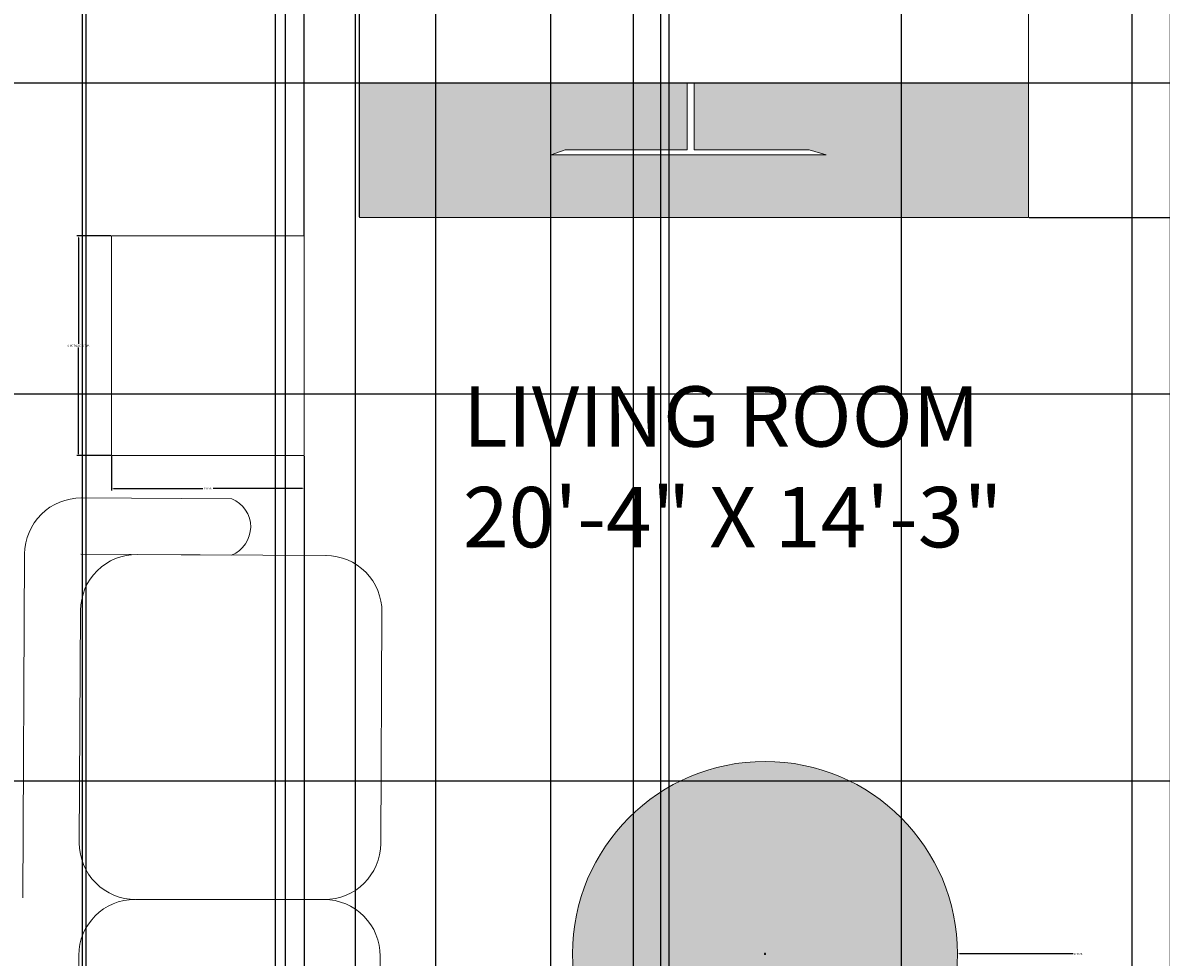
# Model space of a CAD drawing. Units: inches. Extents: x 818 to 1898, y 976 to 2364.
# Tile 34 of 96: x 1278 to 1391, y 1780 to 1873. Entities that reach past the tile are written whole.
import ezdxf

# ---------------------------------------------------------------- set-up
doc = ezdxf.new("R2010")
doc.units = ezdxf.units.IN
doc.header["$LTSCALE"] = 5
doc.header["$MEASUREMENT"] = 0
for name, color, linetype, lineweight in [('A-ANNO-DIMS', 2, 'Continuous', 18), ('A-AREA-IDEN', 7, 'Continuous', 18), ('A-EQPM', 8, 'Continuous', 18), ('A-FLOR-CASE', 8, 'Continuous', 18), ('A-FLOR-CASE-PATT', 33, 'Continuous', 9), ('A-FURN', 8, 'Continuous', 18)]:
    doc.layers.add(name, color=color, linetype=linetype, lineweight=lineweight)
doc.styles.get("Standard").update_dxf_attribs({"font": 'arial.ttf'})
doc.dimstyles.get("Standard").update_dxf_attribs({"dimtxt": 0.18, "dimasz": 0.18, "dimexe": 0.18, "dimexo": 0.0625, "dimgap": 0.09, "dimtad": 0, "dimtih": 1, "dimtoh": 1, "dimdec": 4, "dimzin": 0, "dimdsep": 46, "dimtxsty": 'Standard', "dimcen": 0.09, "dimadec": 0, "dimazin": 0, "dimtfac": 1, "dimtdec": 4, "dimtofl": 0, "dimtmove": 0, "dimatfit": 3, "dimfxl": 1, "dimtolj": 1, "dimtzin": 0, "dimarcsym": 0})

# ---------------------------------------------------------------- blocks, each defined once
blk = doc.blocks.new('SOFA-3-SEAT')
for p, q in [((108.23, 35.49), (74.06, 35.68)), ((68.34, 30.12), (45.43, 30.24)), ((102.62, 29.94), (79.51, 30.06)), ((108.12, 14.94), (108.2, 29.9)), ((113.71, 14.91), (113.79, 29.87)), ((73.9, 5.71), (73.9, 24.47)), ((108.07, 5.56), (108.17, 24.32)), ((45.27, 0.31), (68.27, 0.19)), ((79.45, 0.12), (102.45, 0))]:
    blk.add_line(p, q)
for centre, radius, start, end in [((108.2, 29.9), 5.59, 359.6898, 89.6898), ((68.31, 24.53), 5.59, 0, 89.6898), ((79.48, 24.47), 5.59, 89.6898, 180), ((102.59, 24.35), 5.59, 359.6898, 89.6898), ((110.92, 16.05), 3.01, 201.7034, 337.6762), ((68.3, 5.77), 5.59, 269.6898, 359.6898), ((79.48, 5.71), 5.59, 179.6898, 269.6898), ((102.48, 5.59), 5.59, 269.6898, 359.6898)]:
    blk.add_arc(centre, radius, start, end)
blk = doc.blocks.new('SIDE-TABLE')
blk.add_lwpolyline([(0, 19.12), (21.82, 19.12), (21.82, 0), (0, 0)], close=True)
blk = doc.blocks.new('*D44')
at = {"layer": 'A-ANNO-DIMS', "color": 0, "lineweight": -2, "ltscale": 5, "transparency": 16777216}
for p, q in [((1286.64, 1851.91), (1283.25, 1851.91)), ((1283.43, 1851.73), (1283.43, 1841.18)), ((1283.43, 1830.26), (1283.43, 1840.81)), ((1286.64, 1830.08), (1283.25, 1830.08))]:
    blk.add_line(p, q, dxfattribs=at)
at = {"layer": 'A-ANNO-DIMS', "color": 0, "ltscale": 5, "transparency": 16777216}
for points in [[(1283.4, 1851.73), (1283.46, 1851.73), (1283.43, 1851.91)], [(1283.4, 1830.26), (1283.46, 1830.26), (1283.43, 1830.08)]]:
    blk.add_solid(points, dxfattribs=at)
at = {"layer": 'Defpoints', "color": 0, "ltscale": 5, "transparency": 16777216}
for p in [(1283.43, 1851.91), (1286.7, 1851.91), (1286.7, 1830.08)]:
    blk.add_point(p, dxfattribs=at)
at = {"layer": 'A-ANNO-DIMS', "color": 0, "ltscale": 5, "transparency": 16777216, "insert": (1283.43, 1841), "char_height": 0.18, "attachment_point": 5}
blk.add_mtext('\\A1;SIDE TABLE 22 TYP.', dxfattribs=at)
blk = doc.blocks.new('*D45')
at = {"layer": 'A-ANNO-DIMS', "color": 0, "lineweight": -2, "ltscale": 5, "transparency": 16777216}
for p, q in [((1286.7, 1830.02), (1286.7, 1826.63)), ((1305.83, 1830.02), (1305.83, 1826.63)), ((1286.88, 1826.81), (1295.75, 1826.81)), ((1305.65, 1826.81), (1296.79, 1826.81))]:
    blk.add_line(p, q, dxfattribs=at)
at = {"layer": 'A-ANNO-DIMS', "color": 0, "ltscale": 5, "transparency": 16777216}
for points in [[(1286.88, 1826.84), (1286.88, 1826.78), (1286.7, 1826.81)], [(1305.65, 1826.84), (1305.65, 1826.78), (1305.83, 1826.81)]]:
    blk.add_solid(points, dxfattribs=at)
at = {"layer": 'Defpoints', "color": 0, "ltscale": 5, "transparency": 16777216}
for p in [(1286.7, 1830.08), (1305.83, 1830.08), (1286.7, 1826.81)]:
    blk.add_point(p, dxfattribs=at)
at = {"layer": 'A-ANNO-DIMS', "color": 0, "ltscale": 5, "transparency": 16777216, "insert": (1296.27, 1826.81), "char_height": 0.18, "attachment_point": 5}
blk.add_mtext('\\A1;19 TYP.', dxfattribs=at)
blk = doc.blocks.new('*D61')
at = {"layer": 'A-ANNO-DIMS', "color": 0, "lineweight": -2, "ltscale": 5, "transparency": 16777216}
for p, q in [((1071.73, 1203.03), (1071.73, 2363.87)), ((1071.91, 2363.69), (1250.94, 2363.69)), ((1430.55, 2363.69), (1251.51, 2363.69)), ((1430.73, 1203.03), (1430.73, 2363.87))]:
    blk.add_line(p, q, dxfattribs=at)
at = {"layer": 'A-ANNO-DIMS', "color": 0, "ltscale": 5, "transparency": 16777216}
for points in [[(1071.91, 2363.72), (1071.91, 2363.66), (1071.73, 2363.69)], [(1430.55, 2363.72), (1430.55, 2363.66), (1430.73, 2363.69)]]:
    blk.add_solid(points, dxfattribs=at)
at = {"layer": 'Defpoints', "color": 0, "ltscale": 5, "transparency": 16777216}
for p in [(1430.73, 2363.69), (1071.73, 1202.96), (1430.73, 1202.96)]:
    blk.add_point(p, dxfattribs=at)
at = {"layer": 'A-ANNO-DIMS', "color": 0, "ltscale": 5, "transparency": 16777216, "insert": (1251.23, 2363.69), "char_height": 0.18, "attachment_point": 5}
blk.add_mtext('\\A1;359', dxfattribs=at)
blk = doc.blocks.new('*D64')
at = {"layer": 'A-ANNO-DIMS', "color": 0, "lineweight": -2, "ltscale": 5, "transparency": 16777216}
for p, q in [((1197.73, 1501.14), (1197.73, 2363.87)), ((1197.91, 2363.69), (1313.93, 2363.69)), ((1430.55, 2363.69), (1314.52, 2363.69)), ((1430.73, 1501.14), (1430.73, 2363.87))]:
    blk.add_line(p, q, dxfattribs=at)
at = {"layer": 'A-ANNO-DIMS', "color": 0, "ltscale": 5, "transparency": 16777216}
for points in [[(1197.91, 2363.72), (1197.91, 2363.66), (1197.73, 2363.69)], [(1430.55, 2363.72), (1430.55, 2363.66), (1430.73, 2363.69)]]:
    blk.add_solid(points, dxfattribs=at)
at = {"layer": 'Defpoints', "color": 0, "ltscale": 5, "transparency": 16777216}
for p in [(1430.73, 2363.69), (1197.73, 1501.08), (1430.73, 1501.08)]:
    blk.add_point(p, dxfattribs=at)
at = {"layer": 'A-ANNO-DIMS', "color": 0, "ltscale": 5, "transparency": 16777216, "insert": (1314.23, 2363.69), "char_height": 0.18, "attachment_point": 5}
blk.add_mtext('\\A1;233', dxfattribs=at)
blk = doc.blocks.new('*D85')
at = {"layer": 'A-ANNO-DIMS', "color": 0, "lineweight": -2, "ltscale": 5, "transparency": 16777216}
for p, q in [((1258.79, 2053.08), (1897.92, 2053.08)), ((1897.74, 2052.9), (1897.74, 1876.76)), ((1897.74, 1700.26), (1897.74, 1876.4)), ((1258.79, 1700.08), (1897.92, 1700.08))]:
    blk.add_line(p, q, dxfattribs=at)
at = {"layer": 'A-ANNO-DIMS', "color": 0, "ltscale": 5, "transparency": 16777216}
for points in [[(1897.71, 2052.9), (1897.77, 2052.9), (1897.74, 2053.08)], [(1897.71, 1700.26), (1897.77, 1700.26), (1897.74, 1700.08)]]:
    blk.add_solid(points, dxfattribs=at)
at = {"layer": 'Defpoints', "color": 0, "ltscale": 5, "transparency": 16777216}
for p in [(1258.73, 2053.08), (1897.74, 2053.08), (1258.73, 1700.08)]:
    blk.add_point(p, dxfattribs=at)
at = {"layer": 'A-ANNO-DIMS', "color": 0, "ltscale": 5, "transparency": 16777216, "insert": (1897.74, 1876.58), "char_height": 0.18, "attachment_point": 5}
blk.add_mtext('\\A1;353', dxfattribs=at)
blk = doc.blocks.new('*D96')
at = {"layer": 'A-ANNO-DIMS', "color": 0, "lineweight": -2, "ltscale": 5, "transparency": 16777216}
for p, q in [((1229.65, 1071.12), (1229.65, 2363.87)), ((1229.83, 2363.69), (1256.52, 2363.69)), ((1283.99, 2363.69), (1257.3, 2363.69)), ((1284.17, 1071.12), (1284.17, 2363.87))]:
    blk.add_line(p, q, dxfattribs=at)
at = {"layer": 'A-ANNO-DIMS', "color": 0, "ltscale": 5, "transparency": 16777216}
for points in [[(1229.83, 2363.72), (1229.83, 2363.66), (1229.65, 2363.69)], [(1283.99, 2363.72), (1283.99, 2363.66), (1284.17, 2363.69)]]:
    blk.add_solid(points, dxfattribs=at)
at = {"layer": 'Defpoints', "color": 0, "ltscale": 5, "transparency": 16777216}
for p in [(1284.17, 2363.69), (1229.65, 1071.06), (1284.17, 1071.06)]:
    blk.add_point(p, dxfattribs=at)
at = {"layer": 'A-ANNO-DIMS', "color": 0, "ltscale": 5, "transparency": 16777216, "insert": (1256.91, 2363.69), "char_height": 0.18, "attachment_point": 5}
blk.add_mtext('\\A1;54.52', dxfattribs=at)
blk = doc.blocks.new('*D97')
at = {"layer": 'A-ANNO-DIMS', "color": 0, "lineweight": -2, "ltscale": 5, "transparency": 16777216}
for p, q in [((1284.17, 1071.12), (1284.17, 2363.87)), ((1284.35, 2363.69), (1310.96, 2363.69)), ((1338.36, 2363.69), (1311.75, 2363.69)), ((1338.54, 1071.12), (1338.54, 2363.87))]:
    blk.add_line(p, q, dxfattribs=at)
at = {"layer": 'A-ANNO-DIMS', "color": 0, "ltscale": 5, "transparency": 16777216}
for points in [[(1284.35, 2363.72), (1284.35, 2363.66), (1284.17, 2363.69)], [(1338.36, 2363.72), (1338.36, 2363.66), (1338.54, 2363.69)]]:
    blk.add_solid(points, dxfattribs=at)
at = {"layer": 'Defpoints', "color": 0, "ltscale": 5, "transparency": 16777216}
for p in [(1338.54, 2363.69), (1284.17, 1071.06), (1338.54, 1071.06)]:
    blk.add_point(p, dxfattribs=at)
at = {"layer": 'A-ANNO-DIMS', "color": 0, "ltscale": 5, "transparency": 16777216, "insert": (1311.36, 2363.69), "char_height": 0.18, "attachment_point": 5}
blk.add_mtext('\\A1;54.37', dxfattribs=at)
blk = doc.blocks.new('*D98')
at = {"layer": 'A-ANNO-DIMS', "color": 0, "lineweight": -2, "ltscale": 5, "transparency": 16777216}
for p, q in [((1338.54, 1071.12), (1338.54, 2363.87)), ((1338.72, 2363.69), (1364.81, 2363.69)), ((1391.7, 2363.69), (1365.6, 2363.69)), ((1391.88, 1071.12), (1391.88, 2363.87))]:
    blk.add_line(p, q, dxfattribs=at)
at = {"layer": 'A-ANNO-DIMS', "color": 0, "ltscale": 5, "transparency": 16777216}
for points in [[(1338.72, 2363.72), (1338.72, 2363.66), (1338.54, 2363.69)], [(1391.7, 2363.72), (1391.7, 2363.66), (1391.88, 2363.69)]]:
    blk.add_solid(points, dxfattribs=at)
at = {"layer": 'Defpoints', "color": 0, "ltscale": 5, "transparency": 16777216}
for p in [(1391.88, 2363.69), (1338.54, 1071.06), (1391.88, 1071.06)]:
    blk.add_point(p, dxfattribs=at)
at = {"layer": 'A-ANNO-DIMS', "color": 0, "ltscale": 5, "transparency": 16777216, "insert": (1365.21, 2363.69), "char_height": 0.18, "attachment_point": 5}
blk.add_mtext('\\A1;53.33', dxfattribs=at)
blk = doc.blocks.new('*D120')
at = {"layer": 'A-ANNO-DIMS', "color": 0, "lineweight": -2, "ltscale": 5, "transparency": 16777216}
for p, q in [((1766.29, 1797.72), (818.03, 1797.72)), ((818.21, 1797.54), (818.21, 1757.53)), ((818.21, 1717.17), (818.21, 1757.17)), ((1766.29, 1716.99), (818.03, 1716.99))]:
    blk.add_line(p, q, dxfattribs=at)
at = {"layer": 'A-ANNO-DIMS', "color": 0, "ltscale": 5, "transparency": 16777216}
for points in [[(818.18, 1797.54), (818.24, 1797.54), (818.21, 1797.72)], [(818.18, 1717.17), (818.24, 1717.17), (818.21, 1716.99)]]:
    blk.add_solid(points, dxfattribs=at)
at = {"layer": 'Defpoints', "color": 0, "ltscale": 5, "transparency": 16777216}
for p in [(818.21, 1797.72), (1766.35, 1797.72), (1766.35, 1716.99)]:
    blk.add_point(p, dxfattribs=at)
at = {"layer": 'A-ANNO-DIMS', "color": 0, "ltscale": 5, "transparency": 16777216, "insert": (818.21, 1757.35), "char_height": 0.18, "attachment_point": 5}
blk.add_mtext('\\A1;80.73', dxfattribs=at)
blk = doc.blocks.new('*D121')
at = {"layer": 'A-ANNO-DIMS', "color": 0, "lineweight": -2, "ltscale": 5, "transparency": 16777216}
for p, q in [((1766.29, 1884.2), (818.03, 1884.2)), ((818.21, 1884.02), (818.21, 1841.14)), ((818.21, 1797.9), (818.21, 1840.78)), ((1766.29, 1797.72), (818.03, 1797.72))]:
    blk.add_line(p, q, dxfattribs=at)
at = {"layer": 'A-ANNO-DIMS', "color": 0, "ltscale": 5, "transparency": 16777216}
for points in [[(818.18, 1884.02), (818.24, 1884.02), (818.21, 1884.2)], [(818.18, 1797.9), (818.24, 1797.9), (818.21, 1797.72)]]:
    blk.add_solid(points, dxfattribs=at)
at = {"layer": 'Defpoints', "color": 0, "ltscale": 5, "transparency": 16777216}
for p in [(818.21, 1884.2), (1766.35, 1884.2), (1766.35, 1797.72)]:
    blk.add_point(p, dxfattribs=at)
at = {"layer": 'A-ANNO-DIMS', "color": 0, "ltscale": 5, "transparency": 16777216, "insert": (818.21, 1840.96), "char_height": 0.18, "attachment_point": 5}
blk.add_mtext('\\A1;86.49', dxfattribs=at)
blk = doc.blocks.new('*D162')
at = {"layer": 'A-ANNO-DIMS', "color": 0, "lineweight": -2, "ltscale": 5, "transparency": 16777216}
for p, q in [((1429.16, 1876.08), (818.03, 1876.08)), ((818.21, 1875.9), (818.21, 1871.76)), ((818.21, 1867.26), (818.21, 1871.4)), ((1429.16, 1867.08), (818.03, 1867.08))]:
    blk.add_line(p, q, dxfattribs=at)
at = {"layer": 'A-ANNO-DIMS', "color": 0, "ltscale": 5, "transparency": 16777216}
for points in [[(818.18, 1875.9), (818.24, 1875.9), (818.21, 1876.08)], [(818.18, 1867.26), (818.24, 1867.26), (818.21, 1867.08)]]:
    blk.add_solid(points, dxfattribs=at)
at = {"layer": 'Defpoints', "color": 0, "ltscale": 5, "transparency": 16777216}
for p in [(1429.23, 1876.08), (818.21, 1867.08), (1429.23, 1867.08)]:
    blk.add_point(p, dxfattribs=at)
at = {"layer": 'A-ANNO-DIMS', "color": 0, "ltscale": 5, "transparency": 16777216, "insert": (818.21, 1871.58), "char_height": 0.18, "attachment_point": 5}
blk.add_mtext('\\A1;9', dxfattribs=at)
blk = doc.blocks.new('*D165')
at = {"layer": 'A-ANNO-DIMS', "color": 0, "lineweight": -2, "ltscale": 5, "transparency": 16777216}
for p, q in [((1283.82, 1510.14), (1283.82, 2363.87)), ((1284, 2363.69), (1324.09, 2363.69)), ((1364.97, 2363.69), (1324.88, 2363.69)), ((1365.15, 1510.14), (1365.15, 2363.87))]:
    blk.add_line(p, q, dxfattribs=at)
at = {"layer": 'A-ANNO-DIMS', "color": 0, "ltscale": 5, "transparency": 16777216}
for points in [[(1284, 2363.72), (1284, 2363.66), (1283.82, 2363.69)], [(1364.97, 2363.72), (1364.97, 2363.66), (1365.15, 2363.69)]]:
    blk.add_solid(points, dxfattribs=at)
at = {"layer": 'Defpoints', "color": 0, "ltscale": 5, "transparency": 16777216}
for p in [(1365.15, 2363.69), (1283.82, 1510.08), (1365.15, 1510.08)]:
    blk.add_point(p, dxfattribs=at)
at = {"layer": 'A-ANNO-DIMS', "color": 0, "ltscale": 5, "transparency": 16777216, "insert": (1324.48, 2363.69), "char_height": 0.18, "attachment_point": 5}
blk.add_mtext('\\A1;81.33', dxfattribs=at)
blk = doc.blocks.new('*D215')
at = {"layer": 'A-ANNO-DIMS', "color": 0, "lineweight": -2, "ltscale": 5, "transparency": 16777216}
for p, q in [((1590.66, 1876.08), (818.03, 1876.08)), ((818.21, 1875.9), (818.21, 1781.76)), ((818.21, 1687.26), (818.21, 1781.4)), ((1511.66, 1687.08), (818.03, 1687.08))]:
    blk.add_line(p, q, dxfattribs=at)
at = {"layer": 'A-ANNO-DIMS', "color": 0, "ltscale": 5, "transparency": 16777216}
for points in [[(818.18, 1875.9), (818.24, 1875.9), (818.21, 1876.08)], [(818.18, 1687.26), (818.24, 1687.26), (818.21, 1687.08)]]:
    blk.add_solid(points, dxfattribs=at)
at = {"layer": 'Defpoints', "color": 0, "ltscale": 5, "transparency": 16777216}
for p in [(818.21, 1876.08), (1590.73, 1876.08), (1511.73, 1687.08)]:
    blk.add_point(p, dxfattribs=at)
at = {"layer": 'A-ANNO-DIMS', "color": 0, "ltscale": 5, "transparency": 16777216, "insert": (818.21, 1781.58), "char_height": 0.18, "attachment_point": 5}
blk.add_mtext('\\A1;189', dxfattribs=at)
blk = doc.blocks.new('*D227')
at = {"layer": 'A-ANNO-DIMS', "color": 0, "lineweight": -2, "ltscale": 5, "transparency": 16777216}
for p, q in [((1595.66, 1867.08), (818.03, 1867.08)), ((818.21, 1866.9), (818.21, 1851.81)), ((818.21, 1836.36), (818.21, 1851.45)), ((1594.66, 1836.18), (818.03, 1836.18))]:
    blk.add_line(p, q, dxfattribs=at)
at = {"layer": 'A-ANNO-DIMS', "color": 0, "ltscale": 5, "transparency": 16777216}
for points in [[(818.18, 1866.9), (818.24, 1866.9), (818.21, 1867.08)], [(818.18, 1836.36), (818.24, 1836.36), (818.21, 1836.18)]]:
    blk.add_solid(points, dxfattribs=at)
at = {"layer": 'Defpoints', "color": 0, "ltscale": 5, "transparency": 16777216}
for p in [(818.21, 1867.08), (1595.73, 1867.08), (1594.73, 1836.18)]:
    blk.add_point(p, dxfattribs=at)
at = {"layer": 'A-ANNO-DIMS', "color": 0, "ltscale": 5, "transparency": 16777216, "insert": (818.21, 1851.63), "char_height": 0.18, "attachment_point": 5}
blk.add_mtext('\\A1;30.894', dxfattribs=at)
blk = doc.blocks.new('*D231')
at = {"layer": 'A-ANNO-DIMS', "color": 0, "lineweight": -2, "ltscale": 5, "transparency": 16777216}
for p, q in [((1303.93, 1952.98), (1303.93, 975.66)), ((1402.52, 1952.98), (1402.52, 975.66)), ((1304.11, 975.84), (1352.83, 975.84)), ((1402.34, 975.84), (1353.62, 975.84))]:
    blk.add_line(p, q, dxfattribs=at)
at = {"layer": 'A-ANNO-DIMS', "color": 0, "ltscale": 5, "transparency": 16777216}
for points in [[(1304.11, 975.87), (1304.11, 975.81), (1303.93, 975.84)], [(1402.34, 975.87), (1402.34, 975.81), (1402.52, 975.84)]]:
    blk.add_solid(points, dxfattribs=at)
at = {"layer": 'Defpoints', "color": 0, "ltscale": 5, "transparency": 16777216}
for p in [(1303.93, 1953.04), (1402.52, 1953.04), (1402.52, 975.84)]:
    blk.add_point(p, dxfattribs=at)
at = {"layer": 'A-ANNO-DIMS', "color": 0, "ltscale": 5, "transparency": 16777216, "insert": (1353.22, 975.84), "char_height": 0.18, "attachment_point": 5}
blk.add_mtext('\\A1;98.59', dxfattribs=at)
blk = doc.blocks.new('*D233')
at = {"layer": 'A-ANNO-DIMS', "color": 0, "lineweight": -2, "ltscale": 5, "transparency": 16777216}
for p, q in [((1267.73, 2044.02), (1267.73, 975.66)), ((1303.93, 2008.33), (1303.93, 975.66)), ((1267.91, 975.84), (1285.36, 975.84)), ((1303.75, 975.84), (1286.29, 975.84))]:
    blk.add_line(p, q, dxfattribs=at)
at = {"layer": 'A-ANNO-DIMS', "color": 0, "ltscale": 5, "transparency": 16777216}
for points in [[(1267.91, 975.87), (1267.91, 975.81), (1267.73, 975.84)], [(1303.75, 975.87), (1303.75, 975.81), (1303.93, 975.84)]]:
    blk.add_solid(points, dxfattribs=at)
at = {"layer": 'Defpoints', "color": 0, "ltscale": 5, "transparency": 16777216}
for p in [(1267.73, 2044.08), (1303.93, 2008.39), (1303.93, 975.84)]:
    blk.add_point(p, dxfattribs=at)
at = {"layer": 'A-ANNO-DIMS', "color": 0, "ltscale": 5, "transparency": 16777216, "insert": (1285.83, 975.84), "char_height": 0.18, "attachment_point": 5}
blk.add_mtext('\\A1;36.206', dxfattribs=at)
blk = doc.blocks.new('*D236')
at = {"layer": 'A-ANNO-DIMS', "color": 0, "lineweight": -2, "ltscale": 5, "transparency": 16777216}
for p, q in [((1310.91, 2026.14), (1310.91, 975.66)), ((1342.04, 2026.14), (1342.04, 975.66)), ((1311.09, 975.84), (1326.08, 975.84)), ((1341.86, 975.84), (1326.87, 975.84))]:
    blk.add_line(p, q, dxfattribs=at)
at = {"layer": 'A-ANNO-DIMS', "color": 0, "ltscale": 5, "transparency": 16777216}
for points in [[(1311.09, 975.87), (1311.09, 975.81), (1310.91, 975.84)], [(1341.86, 975.87), (1341.86, 975.81), (1342.04, 975.84)]]:
    blk.add_solid(points, dxfattribs=at)
at = {"layer": 'Defpoints', "color": 0, "ltscale": 5, "transparency": 16777216}
for p in [(1310.91, 2026.21), (1342.04, 2026.21), (1342.04, 975.84)]:
    blk.add_point(p, dxfattribs=at)
at = {"layer": 'A-ANNO-DIMS', "color": 0, "ltscale": 5, "transparency": 16777216, "insert": (1326.48, 975.84), "char_height": 0.18, "attachment_point": 5}
blk.add_mtext('\\A1;31.14', dxfattribs=at)
blk = doc.blocks.new('*D252')
at = {"layer": 'A-ANNO-DIMS', "color": 0, "lineweight": -2, "ltscale": 5, "transparency": 16777216}
for p, q in [((1330.3, 2053.02), (1330.3, 975.66)), ((1388.03, 2053.02), (1388.03, 975.66)), ((1330.48, 975.84), (1358.77, 975.84)), ((1387.85, 975.84), (1359.56, 975.84))]:
    blk.add_line(p, q, dxfattribs=at)
at = {"layer": 'A-ANNO-DIMS', "color": 0, "ltscale": 5, "transparency": 16777216}
for points in [[(1330.48, 975.87), (1330.48, 975.81), (1330.3, 975.84)], [(1387.85, 975.87), (1387.85, 975.81), (1388.03, 975.84)]]:
    blk.add_solid(points, dxfattribs=at)
at = {"layer": 'Defpoints', "color": 0, "ltscale": 5, "transparency": 16777216}
for p in [(1330.3, 2053.08), (1388.03, 2053.08), (1388.03, 975.84)]:
    blk.add_point(p, dxfattribs=at)
at = {"layer": 'A-ANNO-DIMS', "color": 0, "ltscale": 5, "transparency": 16777216, "insert": (1359.17, 975.84), "char_height": 0.18, "attachment_point": 5}
blk.add_mtext('\\A1;57.73', dxfattribs=at)
blk = doc.blocks.new('*D254')
at = {"layer": 'A-ANNO-DIMS', "color": 0, "lineweight": -2, "ltscale": 5, "transparency": 16777216}
for p, q in [((1267.73, 2044.02), (1267.73, 975.66)), ((1330.3, 2044.02), (1330.3, 975.66)), ((1267.91, 975.84), (1298.62, 975.84)), ((1330.12, 975.84), (1299.41, 975.84))]:
    blk.add_line(p, q, dxfattribs=at)
at = {"layer": 'A-ANNO-DIMS', "color": 0, "ltscale": 5, "transparency": 16777216}
for points in [[(1267.91, 975.87), (1267.91, 975.81), (1267.73, 975.84)], [(1330.12, 975.87), (1330.12, 975.81), (1330.3, 975.84)]]:
    blk.add_solid(points, dxfattribs=at)
at = {"layer": 'Defpoints', "color": 0, "ltscale": 5, "transparency": 16777216}
for p in [(1267.73, 2044.08), (1330.3, 2044.08), (1330.3, 975.84)]:
    blk.add_point(p, dxfattribs=at)
at = {"layer": 'A-ANNO-DIMS', "color": 0, "ltscale": 5, "transparency": 16777216, "insert": (1299.02, 975.84), "char_height": 0.18, "attachment_point": 5}
blk.add_mtext('\\A1;62.58', dxfattribs=at)
blk = doc.blocks.new('*D269')
at = {"layer": 'A-ANNO-DIMS', "color": 0, "lineweight": -2, "ltscale": 5, "transparency": 16777216}
for p, q in [((1246.94, 1534.14), (1246.94, 2363.87)), ((1247.12, 2363.69), (1293.71, 2363.69)), ((1341.08, 2363.69), (1294.49, 2363.69)), ((1341.26, 1534.14), (1341.26, 2363.87))]:
    blk.add_line(p, q, dxfattribs=at)
at = {"layer": 'A-ANNO-DIMS', "color": 0, "ltscale": 5, "transparency": 16777216}
for points in [[(1247.12, 2363.72), (1247.12, 2363.66), (1246.94, 2363.69)], [(1341.08, 2363.72), (1341.08, 2363.66), (1341.26, 2363.69)]]:
    blk.add_solid(points, dxfattribs=at)
at = {"layer": 'Defpoints', "color": 0, "ltscale": 5, "transparency": 16777216}
for p in [(1341.26, 2363.69), (1246.94, 1534.08), (1341.26, 1534.08)]:
    blk.add_point(p, dxfattribs=at)
at = {"layer": 'A-ANNO-DIMS', "color": 0, "ltscale": 5, "transparency": 16777216, "insert": (1294.1, 2363.69), "char_height": 0.18, "attachment_point": 5}
blk.add_mtext('\\A1;94.32', dxfattribs=at)
blk = doc.blocks.new('*D275')
at = {"layer": 'A-ANNO-DIMS', "color": 0, "lineweight": -2, "ltscale": 5, "transparency": 16777216}
for p, q in [((1377.84, 1897.87), (1897.92, 1897.87)), ((1897.74, 1897.69), (1897.74, 1875.99)), ((1897.74, 1853.93), (1897.74, 1875.63)), ((1377.84, 1853.75), (1897.92, 1853.75))]:
    blk.add_line(p, q, dxfattribs=at)
at = {"layer": 'A-ANNO-DIMS', "color": 0, "ltscale": 5, "transparency": 16777216}
for points in [[(1897.71, 1897.69), (1897.77, 1897.69), (1897.74, 1897.87)], [(1897.71, 1853.93), (1897.77, 1853.93), (1897.74, 1853.75)]]:
    blk.add_solid(points, dxfattribs=at)
at = {"layer": 'Defpoints', "color": 0, "ltscale": 5, "transparency": 16777216}
for p in [(1377.78, 1897.87), (1897.74, 1897.87), (1377.78, 1853.75)]:
    blk.add_point(p, dxfattribs=at)
at = {"layer": 'A-ANNO-DIMS', "color": 0, "ltscale": 5, "transparency": 16777216, "insert": (1897.74, 1875.81), "char_height": 0.18, "attachment_point": 5}
blk.add_mtext('\\A1;44.12', dxfattribs=at)
blk = doc.blocks.new('*D285')
at = {"layer": 'A-ANNO-DIMS', "color": 0, "lineweight": -2, "ltscale": 5, "transparency": 16777216}
for p, q in [((1305.83, 1830.02), (1305.83, 975.66)), ((1267.73, 1814.9), (1267.73, 975.66)), ((1267.91, 975.84), (1286.47, 975.84)), ((1305.65, 975.84), (1287.08, 975.84))]:
    blk.add_line(p, q, dxfattribs=at)
at = {"layer": 'A-ANNO-DIMS', "color": 0, "ltscale": 5, "transparency": 16777216}
for points in [[(1267.91, 975.87), (1267.91, 975.81), (1267.73, 975.84)], [(1305.65, 975.87), (1305.65, 975.81), (1305.83, 975.84)]]:
    blk.add_solid(points, dxfattribs=at)
at = {"layer": 'Defpoints', "color": 0, "ltscale": 5, "transparency": 16777216}
for p in [(1305.83, 1830.08), (1267.73, 1814.97), (1267.73, 975.84)]:
    blk.add_point(p, dxfattribs=at)
at = {"layer": 'A-ANNO-DIMS', "color": 0, "ltscale": 5, "transparency": 16777216, "insert": (1286.78, 975.84), "char_height": 0.18, "attachment_point": 5}
blk.add_mtext('\\A1;38.1', dxfattribs=at)
blk = doc.blocks.new('*D286')
at = {"layer": 'A-ANNO-DIMS', "color": 0, "lineweight": -2, "ltscale": 5, "transparency": 16777216}
for p, q in [((1305.83, 1851.97), (1305.83, 2363.87)), ((1306.01, 2363.69), (1308.18, 2363.69)), ((1311.15, 2363.69), (1308.97, 2363.69)), ((1311.33, 1853.81), (1311.33, 2363.87))]:
    blk.add_line(p, q, dxfattribs=at)
at = {"layer": 'A-ANNO-DIMS', "color": 0, "ltscale": 5, "transparency": 16777216}
for points in [[(1306.01, 2363.72), (1306.01, 2363.66), (1305.83, 2363.69)], [(1311.15, 2363.72), (1311.15, 2363.66), (1311.33, 2363.69)]]:
    blk.add_solid(points, dxfattribs=at)
at = {"layer": 'Defpoints', "color": 0, "ltscale": 5, "transparency": 16777216}
for p in [(1305.83, 2363.69), (1311.33, 1853.75), (1305.83, 1851.91)]:
    blk.add_point(p, dxfattribs=at)
at = {"layer": 'A-ANNO-DIMS', "color": 0, "ltscale": 5, "transparency": 16777216, "insert": (1308.58, 2363.69), "char_height": 0.18, "attachment_point": 5}
blk.add_mtext('\\A1;5.499', dxfattribs=at)
blk = doc.blocks.new('*D290')
at = {"layer": 'A-ANNO-DIMS', "color": 0, "lineweight": -2, "ltscale": 5, "transparency": 16777216}
for p, q in [((1302.98, 1599.43), (1302.98, 2363.87)), ((1303.16, 2363.69), (1310.57, 2363.69)), ((1318.71, 2363.69), (1311.31, 2363.69)), ((1318.89, 1607.83), (1318.89, 2363.87))]:
    blk.add_line(p, q, dxfattribs=at)
at = {"layer": 'A-ANNO-DIMS', "color": 0, "ltscale": 5, "transparency": 16777216}
for points in [[(1303.16, 2363.72), (1303.16, 2363.66), (1302.98, 2363.69)], [(1318.71, 2363.72), (1318.71, 2363.66), (1318.89, 2363.69)]]:
    blk.add_solid(points, dxfattribs=at)
at = {"layer": 'Defpoints', "color": 0, "ltscale": 5, "transparency": 16777216}
for p in [(1318.89, 2363.69), (1318.89, 1607.77), (1302.98, 1599.37)]:
    blk.add_point(p, dxfattribs=at)
at = {"layer": 'A-ANNO-DIMS', "color": 0, "ltscale": 5, "transparency": 16777216, "insert": (1310.94, 2363.69), "char_height": 0.18, "attachment_point": 5}
blk.add_mtext('\\A1;15.91', dxfattribs=at)
blk = doc.blocks.new('*D292')
at = {"layer": 'A-ANNO-DIMS', "color": 0, "lineweight": -2, "ltscale": 5, "transparency": 16777216}
for p, q in [((1351.51, 1780.57), (1351.69, 1780.57)), ((1351.6, 1780.48), (1351.6, 1780.66)), ((1382.19, 1780.57), (1370.9, 1780.57))]:
    blk.add_line(p, q, dxfattribs=at)
at = {"layer": 'A-ANNO-DIMS', "color": 0, "ltscale": 5, "transparency": 16777216}
blk.add_solid([(1370.9, 1780.6), (1370.9, 1780.54), (1370.72, 1780.57)], dxfattribs=at)
at = {"layer": 'Defpoints', "color": 0, "ltscale": 5, "transparency": 16777216}
for p in [(1332.48, 1780.57), (1370.72, 1780.57)]:
    blk.add_point(p, dxfattribs=at)
at = {"layer": 'A-ANNO-DIMS', "color": 0, "ltscale": 5, "transparency": 16777216, "insert": (1382.68, 1780.57), "char_height": 0.18, "attachment_point": 5}
blk.add_mtext('\\A1;∅38.24', dxfattribs=at)

msp = doc.modelspace()

# ---------------------------------------------------------------- hatches: boundary and pattern name
at = {"layer": 'A-FLOR-CASE-PATT', "ltscale": 5}
h = msp.add_hatch(color=256, dxfattribs=at)
h.dxf.hatch_style = 1
h.paths.add_polyline_path([(1705.7252, 1941.0782), (1681.7252, 1941.0782), (1681.7252, 1900.0782), (1599.7252, 1900.0782), (1599.7252, 1876.0782), (1705.7252, 1876.0782)])
h.paths.add_polyline_path([(1457.7252, 1409.1177), (1457.7252, 1526.6712), (1439.7252, 1526.6712), (1439.7252, 1457.5313), (1446.3307, 1457.5313), (1446.3307, 1468.9514), (1446.8307, 1470.665), (1446.8307, 1469.665), (1446.8307, 1468.9514), (1446.8307, 1456.8361), (1446.8307, 1444.7258), (1446.8307, 1443.3338), (1446.3307, 1444.7258), (1446.3307, 1456.8361), (1439.7252, 1456.8361), (1439.7252, 1355.0782), (1463.7252, 1355.0782), (1463.7252, 1367.3287), (1458.0475, 1367.3287, -0.23606798), (1457.0475, 1369.3287), (1456.0475, 1369.3287, -0.11764706), (1456.0475, 1386.3287), (1457.0475, 1386.3287, -0.23606798), (1458.0475, 1388.3287), (1463.7252, 1388.3287), (1463.7252, 1389.3211)])
h.paths.add_polyline_path([(1341.2593, 1534.0782), (1246.9377, 1534.0782), (1246.9377, 1510.0782), (1341.2593, 1510.0782)])
h.paths.add_polyline_path([(1288.8272, 1519.927), (1289.8272, 1519.927), (1290.5408, 1519.927), (1302.6561, 1519.927), (1314.7664, 1519.927), (1316.1584, 1519.927), (1314.7664, 1519.427), (1302.6561, 1519.427), (1302.6561, 1512.8214), (1301.9609, 1512.8214), (1301.9609, 1519.427), (1290.5408, 1519.427)], flags=16)
h.paths.add_polyline_path([(1377.7791, 1867.0782), (1344.5531, 1867.0782), (1344.5531, 1860.4726), (1355.9731, 1860.4726), (1357.6867, 1859.9726), (1356.6867, 1859.9726), (1355.9731, 1859.9726), (1343.8579, 1859.9726), (1331.7475, 1859.9726), (1330.3556, 1859.9726), (1331.7475, 1860.4726), (1343.8579, 1860.4726), (1343.8579, 1867.0782), (1311.3271, 1867.0782), (1311.3271, 1853.7496), (1377.7791, 1853.7496)])
h.paths.add_polyline_path([(1301.148, 1610.7299, -0.46196039), (1314.4882, 1599.3725, -0.19222541), (1311.3254, 1591.4497, 0.54791519), (1336.8832, 1607.7707, 0.92061359)])
h.paths.add_polyline_path([(1370.719, 1780.5695, 1), (1332.478, 1780.5695, 1)])
h.paths.add_polyline_path([(1705.7252, 1463.0782), (1681.7252, 1463.0782), (1681.7252, 1379.0782), (1622.7252, 1379.0782), (1622.7252, 1355.0782), (1705.7252, 1355.0782)])
h.paths.add_polyline_path([(1658.1052, 1359.2188), (1658.1786, 1359.2188), (1658.1786, 1373.8763), (1658.1052, 1373.9202)], flags=16)
h.paths.add_polyline_path([(1686.9271, 1409.9311), (1686.8832, 1409.8578), (1701.5845, 1409.8578), (1701.5845, 1409.9311)], flags=16)
h.paths.add_polyline_path([(1637.1266, 1359.2188), (1637.2, 1359.2188), (1637.2, 1373.8763), (1637.1266, 1373.9202)], flags=16)

# ---------------------------------------------------------------- linework, layer by layer
at = {"layer": 'A-EQPM'}
for p, q in [((1330.3556, 1859.9726), (1331.7475, 1860.4726)), ((1343.8579, 1860.4726), (1331.7475, 1860.4726)), ((1344.5531, 1860.4726), (1355.9731, 1860.4726)), ((1357.6867, 1859.9726), (1355.9731, 1860.4726)), ((1331.7475, 1859.9726), (1330.3556, 1859.9726)), ((1343.8579, 1859.9726), (1331.7475, 1859.9726)), ((1343.8579, 1859.9726), (1355.9731, 1859.9726)), ((1355.9731, 1859.9726), (1356.6867, 1859.9726)), ((1356.6867, 1859.9726), (1357.6867, 1859.9726))]:
    msp.add_line(p, q, dxfattribs=at)
msp.add_lwpolyline([(1343.8579, 1860.4726), (1343.8579, 1867.0782), (1344.5531, 1867.0782), (1344.5531, 1860.4726)], dxfattribs=at)
at = {"layer": 'A-FLOR-CASE'}
for p, q in [((1311.3271, 1876.0782), (1311.3271, 1867.0782)), ((1377.7791, 1876.0782), (1377.7791, 1867.0782)), ((1377.7791, 1867.0782), (1311.3271, 1867.0782)), ((1311.3271, 1867.0782), (1311.3271, 1853.7496)), ((1377.7791, 1867.0782), (1377.7791, 1853.7496)), ((1311.3271, 1853.7496), (1377.7791, 1853.7496))]:
    msp.add_line(p, q, dxfattribs=at)
at = {"layer": 'A-FURN'}
msp.add_circle((1351.5985, 1780.5695), 19.1205, dxfattribs=at)

# ---------------------------------------------------------------- block references
for name, p, rotation in [('SIDE-TABLE', (1305.8276, 1830.0849), 90.00000000000014), ('SOFA-3-SEAT', (1313.5566, 1712.0791), 90.0000000000007)]:
    msp.add_blockref(name, p, dxfattribs=dict(at, rotation=rotation))

# ---------------------------------------------------------------- texts
at = {"layer": 'A-AREA-IDEN', "ltscale": 5, "insert": (1321.5948, 1836.9692), "char_height": 6, "attachment_point": 1}
msp.add_mtext_dynamic_manual_height_columns('LIVING ROOM\\P20\'-4" X 14\'-3"', width=118.992422, gutter_width=1, heights=[0], dxfattribs=at)

# ---------------------------------------------------------------- dimensions: what is measured, and where the dimension line sits
at = {"layer": 'A-ANNO-DIMS', "ltscale": 5}
for base, p1, p2, override, picture, middle in [((1430.7251, 2363.6929), (1071.7251, 1202.9642), (1430.7251, 1202.9642), {"dimdec": 0, "dimlfac": 1, "dimrnd": 0, "dimzin": 0, "dimdsep": 46, "dimlunit": 2}, '*D61', (1251.2251, 2363.6929)), ((1430.7251, 2363.6929), (1197.7251, 1501.0782), (1430.7251, 1501.0782), {"dimdec": 0, "dimlfac": 1, "dimrnd": 0, "dimzin": 0, "dimdsep": 46, "dimlunit": 2}, '*D64', (1314.2251, 2363.6929)), ((1284.1697, 2363.6929), (1229.6474, 1071.0552), (1284.1697, 1071.0552), {"dimdec": 2, "dimlfac": 1, "dimrnd": 0, "dimzin": 0, "dimdsep": 46, "dimlunit": 2}, '*D96', (1256.9085, 2363.6929)), ((1341.2593, 2363.6929), (1246.9377, 1534.0782), (1341.2593, 1534.0782), {"dimdec": 2, "dimlfac": 1, "dimrnd": 0, "dimzin": 0, "dimdsep": 46, "dimlunit": 2}, '*D269', (1294.0985, 2363.6929)), ((1365.1463, 2363.6929), (1283.8183, 1510.0782), (1365.1463, 1510.0782), {"dimdec": 2, "dimlfac": 1, "dimrnd": 0, "dimzin": 0, "dimdsep": 46, "dimlunit": 2}, '*D165', (1324.4823, 2363.6929)), ((1338.5412, 2363.6929), (1284.1697, 1071.0552), (1338.5412, 1071.0552), {"dimdec": 2, "dimlfac": 1, "dimrnd": 0, "dimzin": 0, "dimdsep": 46, "dimlunit": 2}, '*D97', (1311.3554, 2363.6929)), ((1318.8931, 2363.6929), (1302.9835, 1599.3725), (1318.8931, 1607.7707), {"dimdec": 2, "dimlfac": 1, "dimrnd": 0, "dimzin": 0, "dimdsep": 46, "dimlunit": 2}, '*D290', (1310.9383, 2363.6929)), ((1305.8278, 2363.6929), (1311.3271, 1853.7496), (1305.8278, 1851.9081), {"dimdec": 3, "dimlfac": 1, "dimrnd": 0, "dimzin": 0, "dimdsep": 46, "dimlunit": 2}, '*D286', (1308.5774, 2363.6929)), ((1391.8757, 2363.6929), (1338.5412, 1071.0552), (1391.8757, 1071.0552), {"dimdec": 2, "dimlfac": 1, "dimrnd": 0, "dimzin": 0, "dimdsep": 46, "dimlunit": 2}, '*D98', (1365.2084, 2363.6929)), ((1388.0315, 975.8433), (1330.305, 2053.0782), (1388.0315, 2053.0782), {"dimdec": 2, "dimlfac": 1, "dimrnd": 0, "dimzin": 0, "dimdsep": 46, "dimlunit": 2}, '*D252', (1359.1682, 975.8433)), ((1303.9314, 975.8433), (1267.7251, 2044.0782), (1303.9314, 2008.3917), {"dimdec": 3, "dimlfac": 1, "dimrnd": 0, "dimzin": 0, "dimdsep": 46, "dimlunit": 2}, '*D233', (1285.8283, 975.8433)), ((1330.305, 975.8433), (1267.7251, 2044.0782), (1330.305, 2044.0782), {"dimdec": 2, "dimlfac": 1, "dimrnd": 0, "dimzin": 0, "dimdsep": 46, "dimlunit": 2}, '*D254', (1299.0151, 975.8433)), ((1342.0448, 975.8433), (1310.9077, 2026.2074), (1342.0448, 2026.2074), {"dimdec": 2, "dimlfac": 1, "dimrnd": 0, "dimzin": 0, "dimdsep": 46, "dimlunit": 2}, '*D236', (1326.4762, 975.8433)), ((1402.518, 975.8433), (1303.9314, 1953.0408), (1402.518, 1953.0408), {"dimdec": 2, "dimlfac": 1, "dimrnd": 0, "dimzin": 0, "dimdsep": 46, "dimlunit": 2}, '*D231', (1353.2247, 975.8433)), ((1267.7251, 975.8433), (1305.8278, 1830.0844), (1267.7251, 1814.9652), {"dimdec": 1, "dimlfac": 1, "dimrnd": 0, "dimzin": 0, "dimdsep": 46, "dimlunit": 2}, '*D285', (1286.7765, 975.8433))]:
    dim = msp.add_linear_dim(base=base, p1=p1, p2=p2, dimstyle='Standard', override=override, dxfattribs=at)
    dim.commit()
    dim.dimension.update_dxf_attribs({"geometry": picture, "text_midpoint": middle})
for base, p1, p2, override, picture, middle in [((1897.736, 2053.0782), (1258.7251, 1700.0782), (1258.7251, 2053.0782), {"dimdec": 0, "dimlfac": 1, "dimrnd": 0, "dimzin": 0, "dimdsep": 46, "dimlunit": 2}, '*D85', (1897.736, 1876.5782)), ((1897.736, 1897.8663), (1377.7791, 1853.7496), (1377.7791, 1897.8663), {"dimdec": 2, "dimlfac": 1, "dimrnd": 0, "dimzin": 0, "dimdsep": 46, "dimlunit": 2}, '*D275', (1897.736, 1875.808)), ((818.2059, 1884.2031), (1766.3524, 1797.7165), (1766.3524, 1884.2031), {"dimdec": 2, "dimlfac": 1, "dimrnd": 0, "dimzin": 0, "dimdsep": 46, "dimlunit": 2}, '*D121', (818.2059, 1840.9598)), ((818.2059, 1876.0782), (1511.7251, 1687.0782), (1590.7251, 1876.0782), {"dimdec": 0, "dimlfac": 1, "dimrnd": 0, "dimzin": 0, "dimdsep": 46, "dimlunit": 2}, '*D215', (818.2059, 1781.5782)), ((818.2059, 1867.0782), (1429.2251, 1876.0782), (1429.2251, 1867.0782), {"dimdec": 0, "dimlfac": 1, "dimrnd": 0, "dimzin": 0, "dimdsep": 46, "dimlunit": 2}, '*D162', (818.2059, 1871.5782)), ((818.2059, 1867.0782), (1594.7251, 1836.1844), (1595.7251, 1867.0782), {"dimdec": 3, "dimlfac": 1, "dimrnd": 0, "dimzin": 0, "dimdsep": 46, "dimlunit": 2}, '*D227', (818.2059, 1851.6313)), ((818.2059, 1797.7165), (1766.3524, 1716.9866), (1766.3524, 1797.7165), {"dimdec": 2, "dimlfac": 1, "dimrnd": 0, "dimzin": 0, "dimdsep": 46, "dimlunit": 2}, '*D120', (818.2059, 1757.3516))]:
    dim = msp.add_linear_dim(base=base, p1=p1, p2=p2, angle=90, dimstyle='Standard', override=override, dxfattribs=at)
    dim.commit()
    dim.dimension.update_dxf_attribs({"geometry": picture, "text_midpoint": middle})
for base, p1, p2, angle, text, picture, middle in [((1283.4294, 1851.9081), (1286.703, 1830.0844), (1286.703, 1851.9081), 90, 'SIDE TABLE <> TYP.', '*D44', (1283.4294, 1840.9963)), ((1286.703, 1826.8109), (1305.8278, 1830.0844), (1286.703, 1830.0844), 180, '<> TYP.', '*D45', (1296.2654, 1826.8109))]:
    dim = msp.add_linear_dim(base=base, p1=p1, p2=p2, angle=angle, text=text, dimstyle='Standard', override={"dimdec": 0, "dimlfac": 1, "dimrnd": 0, "dimzin": 0, "dimdsep": 46, "dimlunit": 2}, dxfattribs=at)
    dim.commit()
    dim.dimension.update_dxf_attribs({"geometry": picture, "text_midpoint": middle})
dim = msp.add_diameter_dim_2p(p1=(1332.478, 1780.5699), p2=(1370.719, 1780.569), dimstyle='Standard', override={"dimdec": 2, "dimlfac": 1, "dimrnd": 0, "dimzin": 0, "dimdsep": 46, "dimlunit": 2}, dxfattribs=at)
dim.commit()
dim.dimension.update_dxf_attribs({"geometry": '*D292', "text_midpoint": (1382.1913, 1780.5687), "dimtype": 163})

doc.saveas('drawing.dxf')
